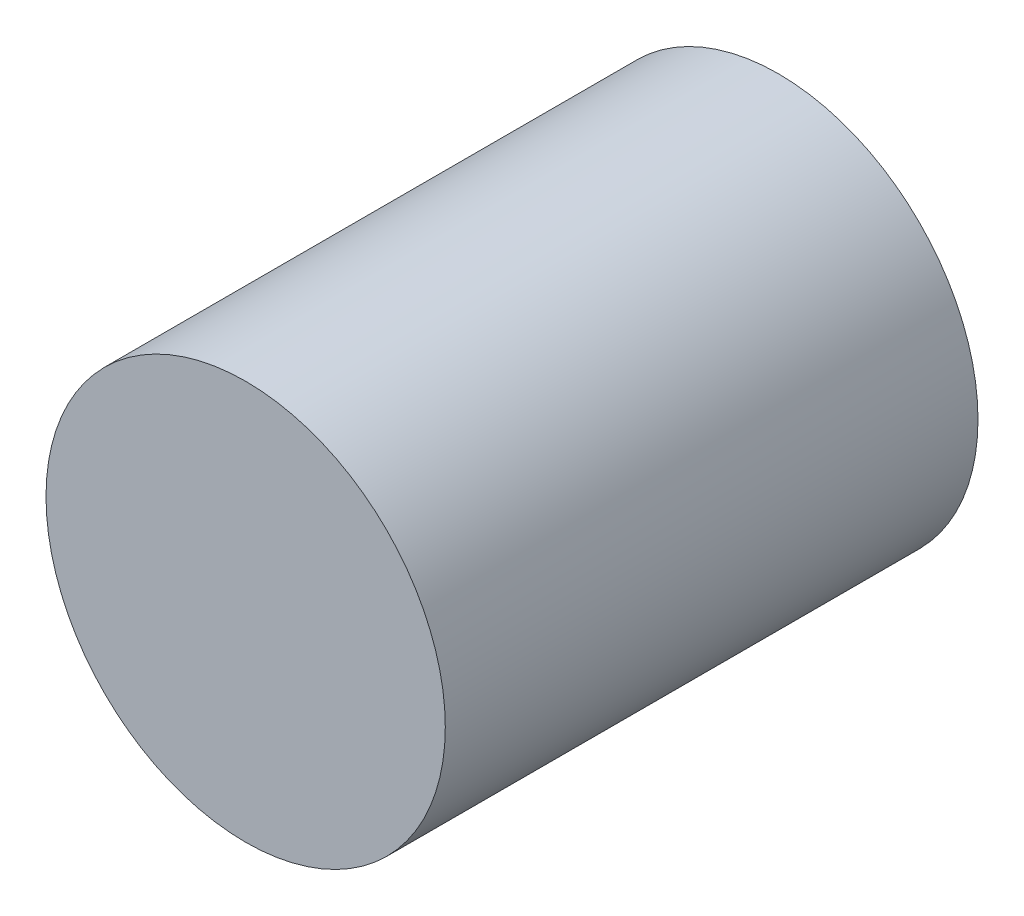
from build123d import *

# Parameters (mm, degrees)
PIN_PROFILE_9_52_R          = 4.76
PIN_BODY_EXTRUDE_12_7_DEPTH = 12.7


with BuildPart() as part:
    # Pin Profile Ø9.52 → Pin Body Extrude 12.7 (new body)
    with BuildSketch(Plane.XY):
        Circle(PIN_PROFILE_9_52_R)
    extrude(amount=PIN_BODY_EXTRUDE_12_7_DEPTH)


solid = part.part
